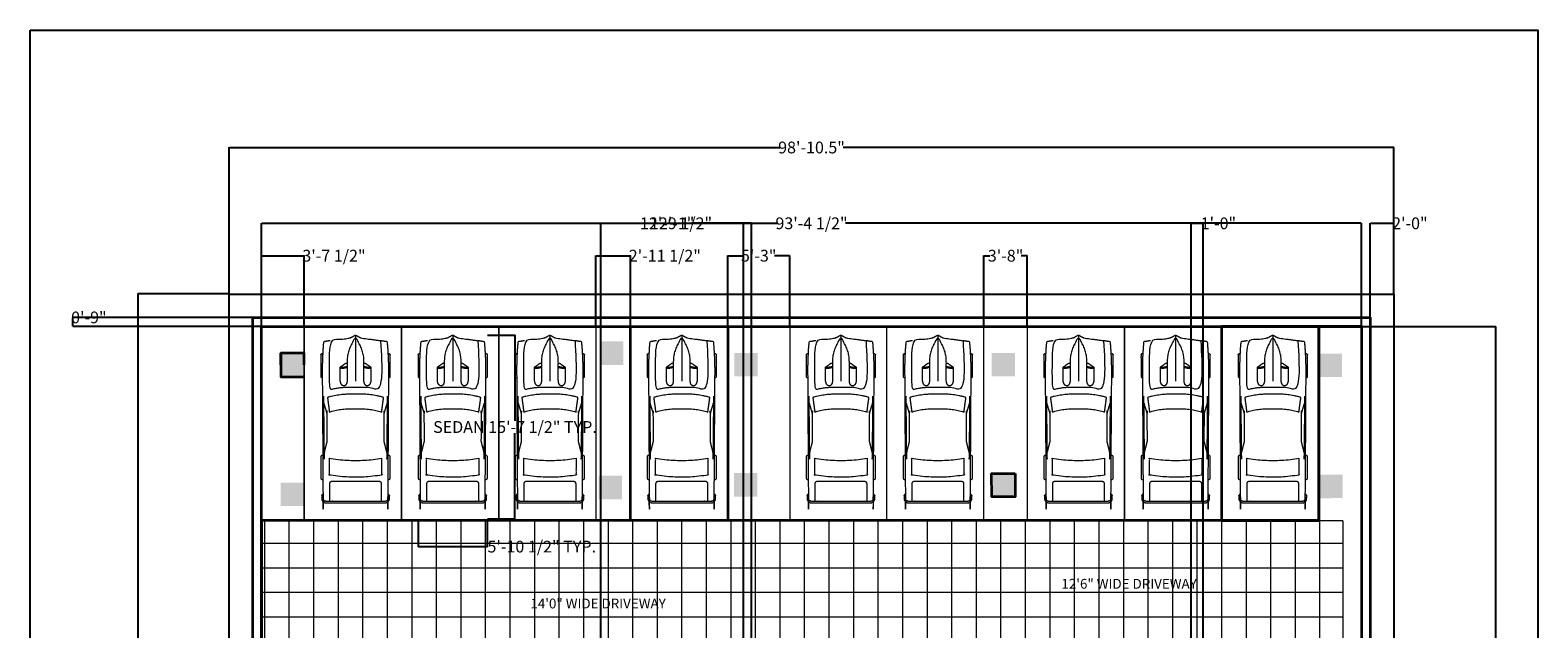
# Model space of a CAD drawing. Units: inches. Extents: x 48986 to 50522, y 132527 to 134098.
# Tile 4 of 4: x 48986 to 50522, y 133488 to 134098. Entities that reach past the tile are written whole.
import ezdxf

# ---------------------------------------------------------------- set-up
doc = ezdxf.new("R2010")
doc.units = ezdxf.units.IN
doc.header["$MEASUREMENT"] = 0
for name, color, linetype, lineweight in [('A-ANNO-DIMS', 2, 'Continuous', 18), ('A-ANNO-TEXT', 7, 'Continuous', 18), ('A-ANNO-TTLB', 7, 'Continuous', 25), ('A-COLS-PATT', 215, 'Continuous', 13), ('A-EQPM-VEHC', 8, 'Continuous', 13), ('A-FLOR-PATT', 94, 'Continuous', 9), ('A-FLOR-PKNG', 140, 'Continuous', 18), ('C-PROP', 160, 'Continuous', 25), ('COLUMNS', 211, 'Continuous', 35), ('WALLS', 140, 'Continuous', 35)]:
    doc.layers.add(name, color=color, linetype=linetype, lineweight=lineweight)
doc.styles.get("Standard").update_dxf_attribs({"font": 'arial.ttf'})
doc.dimstyles.get("Standard").update_dxf_attribs({"dimtxt": 12, "dimasz": 0.18, "dimexe": 0.18, "dimexo": 0.0625, "dimgap": 0.09, "dimtad": 0, "dimtih": 1, "dimtoh": 1, "dimdec": 1, "dimzin": 0, "dimdsep": 46, "dimlunit": 3, "dimtxsty": 'Standard', "dimcen": 0.09, "dimadec": 0, "dimazin": 0, "dimtfac": 1, "dimtdec": 1, "dimtofl": 0, "dimtmove": 0, "dimatfit": 3, "dimfxl": 1, "dimtolj": 1, "dimtzin": 0, "dimarcsym": 0})

# ---------------------------------------------------------------- blocks, each defined once
blk = doc.blocks.new('*D2')
at = {"layer": 'A-ANNO-DIMS', "color": 0, "lineweight": -2, "transparency": 16777216}
for p, q in [((49188.8, 133829.1), (49188.8, 133978.6)), ((49189, 133978.4), (49749.7, 133978.4)), ((50375.1, 133978.4), (49814.4, 133978.4)), ((50375.3, 133829.1), (50375.3, 133978.6))]:
    blk.add_line(p, q, dxfattribs=at)
at = {"layer": 'A-ANNO-DIMS', "color": 0, "transparency": 16777216}
for points in [[(49189, 133978.4), (49189, 133978.4), (49188.8, 133978.4)], [(50375.1, 133978.4), (50375.1, 133978.4), (50375.3, 133978.4)]]:
    blk.add_solid(points, dxfattribs=at)
at = {"layer": 'Defpoints', "color": 0, "transparency": 16777216}
for p in [(50375.3, 133978.4), (49188.8, 133829.1), (50375.3, 133829.1)]:
    blk.add_point(p, dxfattribs=at)
at = {"layer": 'A-ANNO-DIMS', "color": 0, "transparency": 16777216, "insert": (49782, 133978.4), "char_height": 12, "attachment_point": 5}
blk.add_mtext('\\A1;98\'-10.5"', dxfattribs=at)
blk = doc.blocks.new('*D3')
at = {"layer": 'A-ANNO-DIMS', "color": 0, "lineweight": -2, "transparency": 16777216}
for p, q in [((49188.7, 133829.1), (49095.4, 133829.1)), ((49095.6, 133828.9), (49095.6, 133304.8)), ((49095.6, 132768.2), (49095.6, 133292.3)), ((49188.7, 132768.1), (49095.4, 132768.1))]:
    blk.add_line(p, q, dxfattribs=at)
at = {"layer": 'A-ANNO-DIMS', "color": 0, "transparency": 16777216}
for points in [[(49095.6, 133828.9), (49095.6, 133828.9), (49095.6, 133829.1)], [(49095.6, 132768.2), (49095.6, 132768.2), (49095.6, 132768.1)]]:
    blk.add_solid(points, dxfattribs=at)
at = {"layer": 'Defpoints', "color": 0, "transparency": 16777216}
for p in [(49188.8, 133829.1), (49095.6, 132768.1), (49188.8, 132768.1)]:
    blk.add_point(p, dxfattribs=at)
at = {"layer": 'A-ANNO-DIMS', "color": 0, "transparency": 16777216, "insert": (49095.6, 133298.6), "char_height": 12, "attachment_point": 5}
blk.add_mtext('\\A1;88\'-5.0"', dxfattribs=at)
blk = doc.blocks.new('CAR-SEDAN-PLAN')
for p, q in [((35.3, 177.5), (35.3, 130.6)), ((25.7, 8.4), (44.8, 8.4))]:
    blk.add_line(p, q)
for centre, major_axis, start_param, end_param in [((19.9, 164.6), (-24.9, 0), 1.564964, 1.848039), ((50.7, 164.6), (24.9, 0), 4.435146, 4.718221)]:
    blk.add_ellipse(centre, major_axis=major_axis, ratio=0.842304, start_param=start_param, end_param=end_param)
for points, weights, knots in [([(9.6, 171.8), (6.2, 171.2), (2.7, 170.6), (1.4, 156), (1.4, 141.3)], [1, 0.999923835344, 1, 0.999337806115, 1], [0, 0, 0, 0.02468451, 0.02468451, 0.0974728, 0.0974728, 0.0974728]), ([(60.9, 171.8), (56.4, 172.5), (51.9, 173.1), (46.3, 173.7), (40.8, 174.6), (38.2, 176), (35.7, 177.4), (35.3, 177.6), (34.9, 177.4), (32.3, 176), (29.7, 174.6), (24.2, 173.7), (18.7, 173.1), (14.2, 172.5), (9.6, 171.8), (7.9, 146.8), (9.2, 121.9), (17.2, 123.7), (25.5, 124.1), (35.3, 124.1), (45.1, 124.1), (53.3, 123.7), (61.3, 121.9), (62.7, 146.8), (60.9, 171.8)], [1, 0.999861960732, 1, 0.999699858145, 1, 1, 1, 0.835952709181, 1, 1, 1, 0.999699858145, 1, 0.999861960732, 1, 0.998625728423, 1, 0.994860280211, 1, 1, 1, 0.994860280211, 1, 0.998625728423, 1], [0, 0, 0, 0.033232, 0.033232, 0.082234, 0.082234, 1.082234, 1.082234, 2.244094, 2.244094, 3.244094, 3.244094, 3.293097, 3.293097, 3.326328, 3.326328, 3.431193, 3.431193, 3.634055, 3.634055, 4.634055, 4.634055, 4.836917, 4.836917, 4.941783, 4.941783, 4.941783]), ([(43.9, 145.6), (47.3, 144.7), (50.9, 144.8), (50.9, 138), (50.9, 131.3), (50.6, 126), (47.4, 125.7), (44.2, 125.4), (43.9, 130.6), (43.9, 140.6), (43.9, 150.5), (43.9, 163.6), (35.3, 174.4), (26.7, 163.6), (26.7, 150.5), (26.7, 140.6), (26.7, 130.6), (26.4, 125.4), (23.2, 125.7), (20, 126), (19.7, 131.3), (19.7, 138), (19.7, 144.8), (23.3, 144.7), (26.7, 145.6)], [1, 0.990000279832, 1, 1, 1, 0.735618766318, 1, 0.735618766318, 1, 1, 1, 0.956755789522, 1, 0.956755789522, 1, 1, 1, 0.735618766318, 1, 0.735618766318, 1, 1, 1, 0.990000279832, 1], [0, 0, 0, 0.283075, 0.283075, 1.283075, 1.283075, 2.771508, 2.771508, 4.259942, 4.259942, 5.259942, 5.259942, 5.85026, 5.85026, 6.440579, 6.440579, 7.440579, 7.440579, 8.929012, 8.929012, 10.417446, 10.417446, 11.417446, 11.417446, 11.700521, 11.700521, 11.700521]), ([(69.2, 141.3), (69.1, 156), (67.8, 170.6), (64.4, 171.2), (60.9, 171.8)], [1, 0.999337806115, 1, 0.999923835344, 1], [0, 0, 0, 0.07278829, 0.07278829, 0.0974728, 0.0974728, 0.0974728]), ([(1.9, 158.4), (1.6, 158.4), (1.3, 158.4), (0.8, 158.4), (0.4, 158.1), (0, 157.7), (0, 157.3), (0, 146.3), (0, 135.3), (0, 134.8), (0.4, 134.5), (0.8, 134.2), (1.3, 134.2), (1.4, 134.2), (1.4, 134.2)], [1, 1, 1, 0.923879532511, 1, 0.923879532511, 1, 1, 1, 0.923879532511, 1, 0.923879532511, 1, 1, 1], [0, 0, 0, 1, 1, 1.785398, 1.785398, 2.570796, 2.570796, 3.570796, 3.570796, 4.356194, 4.356194, 5.141593, 5.141593, 6.141593, 6.141593, 6.141593]), ([(69.2, 134.2), (69.2, 134.2), (69.2, 134.2), (69.8, 134.2), (70.2, 134.5), (70.6, 134.8), (70.6, 135.3), (70.6, 146.3), (70.6, 157.3), (70.6, 157.7), (70.2, 158.1), (69.8, 158.4), (69.2, 158.4), (69, 158.4), (68.7, 158.4)], [1, 1, 1, 0.923879532511, 1, 0.923879532511, 1, 1, 1, 0.923879532511, 1, 0.923879532511, 1, 1, 1], [0, 0, 0, 1, 1, 1.785398, 1.785398, 2.570796, 2.570796, 3.570796, 3.570796, 4.356194, 4.356194, 5.141593, 5.141593, 6.141593, 6.141593, 6.141593]), ([(1.4, 141.7), (1.2, 76.1), (2.2, 10.6), (2.2, 8.4), (4.9, 8.4), (35.3, 8.4), (65.7, 8.4), (68.3, 8.4), (68.4, 10.6), (69.4, 76.1), (69.2, 141.7)], [1, 0.999967219517, 1, 0.711827418646, 1, 1, 1, 0.711827418646, 1, 0.999967219517, 1], [0, 0, 0, 0.016194, 0.016194, 1.573593, 1.573593, 2.573593, 2.573593, 4.130993, 4.130993, 4.147187, 4.147187, 4.147187]), ([(26.7, 148.4), (25.9, 148.4), (25.2, 148.4), (24.9, 148.4), (24.7, 148.3), (22.2, 146.5), (19.7, 144.8)], [1, 1, 1, 0.940892222322, 1, 1, 1], [0, 0, 0, 1, 1, 1.691083, 1.691083, 2.691083, 2.691083, 2.691083]), ([(50.9, 144.8), (48.3, 146.5), (45.8, 148.3), (45.6, 148.4), (45.4, 148.4), (44.7, 148.4), (43.9, 148.4)], [1, 1, 1, 0.940892222322, 1, 1, 1], [0, 0, 0, 1, 1, 1.691083, 1.691083, 2.691083, 2.691083, 2.691083]), ([(6.5, 69.3), (4.7, 62.5), (3, 55.7), (2.7, 82.7), (2.7, 109.7), (4.5, 103.7), (6.4, 97.7), (6.3, 83.5), (6.5, 69.3)], [1, 1, 1, 0.999994429546, 1, 1, 1, 0.999987377106, 1], [0, 0, 0, 1, 1, 1.006676, 1.006676, 2.006676, 2.006676, 2.016725, 2.016725, 2.016725]), ([(61.9, 99.1), (52.7, 101.9), (43, 102.5), (35.3, 102.5), (27.6, 102.5), (17.8, 101.9), (8.7, 99.1), (7.7, 106.6), (6.7, 114), (16, 116.6), (25.7, 117.2), (35.3, 117.2), (44.8, 117.2), (54.6, 116.6), (63.9, 114), (62.9, 106.6), (61.9, 99.1)], [1, 0.991000078903, 1, 1, 1, 0.991000078903, 1, 1, 1, 0.991394232237, 1, 1, 1, 0.991394232237, 1, 1, 1], [0, 0, 0, 0.268529, 0.268529, 1.268529, 1.268529, 1.537057, 1.537057, 2.537057, 2.537057, 2.799631, 2.799631, 3.799631, 3.799631, 4.062205, 4.062205, 5.062205, 5.062205, 5.062205]), ([(64.1, 69.3), (64.2, 83.5), (64.2, 97.7), (66, 103.7), (67.9, 109.7), (67.8, 82.7), (67.6, 55.7), (65.8, 62.5), (64.1, 69.3)], [1, 0.999987377106, 1, 1, 1, 0.999994429546, 1, 1, 1], [0, 0, 0, 0.010049, 0.010049, 1.010049, 1.010049, 1.016725, 1.016725, 2.016725, 2.016725, 2.016725]), ([(1.7, 54.7), (1.5, 54.7), (1.3, 54.7), (0, 54.7), (0, 53.5), (0, 42.5), (0, 31.6), (0, 30.4), (1.3, 30.4), (1.6, 30.4), (1.9, 30.4)], [1, 1, 1, 0.707106781187, 1, 1, 1, 0.707106781187, 1, 1, 1], [0, 0, 0, 1, 1, 2.570796, 2.570796, 3.570796, 3.570796, 5.141593, 5.141593, 6.141593, 6.141593, 6.141593]), ([(61.9, 52), (35.3, 47.4), (8.7, 52), (8.7, 43.4), (8.7, 34.9), (35.3, 30.3), (61.9, 34.9), (61.9, 43.4), (61.9, 52)], [1, 0.979868494456, 1, 1, 1, 0.979868494456, 1, 1, 1], [0, 0, 0, 0.401989, 0.401989, 1.401989, 1.401989, 1.803978, 1.803978, 2.803978, 2.803978, 2.803978]), ([(68.6, 30.4), (68.9, 30.4), (69.2, 30.4), (69.8, 30.4), (70.2, 30.8), (70.6, 31.1), (70.6, 31.6), (70.6, 42.5), (70.6, 53.5), (70.6, 54), (70.2, 54.3), (69.8, 54.7), (69.2, 54.7), (69.1, 54.7), (68.9, 54.7)], [1, 1, 1, 0.923879532511, 1, 0.923879532511, 1, 1, 1, 0.923879532511, 1, 0.923879532511, 1, 1, 1], [0, 0, 0, 1, 1, 1.785398, 1.785398, 2.570796, 2.570796, 3.570796, 3.570796, 4.356194, 4.356194, 5.141593, 5.141593, 6.141593, 6.141593, 6.141593]), ([(61.9, 8.4), (61.9, 17.2), (61.9, 26), (61.9, 28.3), (59.2, 28.3), (35.3, 28.3), (11.3, 28.3), (8.7, 28.3), (8.7, 26), (8.7, 17.2), (8.7, 8.4)], [1, 1, 1, 0.707106781187, 1, 1, 1, 0.707106781187, 1, 1, 1], [0, 0, 0, 1, 1, 2.570796, 2.570796, 3.570796, 3.570796, 5.141593, 5.141593, 6.141593, 6.141593, 6.141593]), ([(2.1, 15.3), (0.7, 14.9), (0.8, 13.6), (0.8, 12.1), (0.8, 10.6), (0.9, 6.6), (5.6, 6.6), (35.3, 6.6), (65, 6.6), (69.7, 6.6), (69.8, 10.6), (69.8, 12.1), (69.8, 13.6), (69.8, 14.9), (68.4, 15.3)], [1, 0.807168985933, 1, 0.999999981995, 1, 0.711827418646, 1, 1, 1, 0.711827418646, 1, 0.999999981995, 1, 0.807168985459, 1], [0, 0, 0, 1.262912, 1.262912, 1.263291, 1.263291, 2.82069, 2.82069, 3.82069, 3.82069, 5.37809, 5.37809, 5.378469, 5.378469, 6.641381, 6.641381, 6.641381])]:
    blk.add_rational_spline(points, weights, degree=2, knots=knots)
blk = doc.blocks.new('PARKING-STALL-99X198')
blk.add_lwpolyline([(198, 0), (198, 99), (0, 99), (0, 0)], close=True)
blk = doc.blocks.new('*D11')
at = {"layer": 'A-ANNO-DIMS', "color": 0, "lineweight": -2, "transparency": 16777216}
for p, q in [((49451.8, 133787.2), (49480, 133787.2)), ((49479.9, 133787), (49479.9, 133699.8)), ((49479.9, 133599.9), (49479.9, 133687.2)), ((49451.8, 133599.8), (49480, 133599.8))]:
    blk.add_line(p, q, dxfattribs=at)
at = {"layer": 'A-ANNO-DIMS', "color": 0, "transparency": 16777216}
for points in [[(49479.8, 133787), (49479.9, 133787), (49479.9, 133787.2)], [(49479.8, 133599.9), (49479.9, 133599.9), (49479.9, 133599.8)]]:
    blk.add_solid(points, dxfattribs=at)
at = {"layer": 'Defpoints', "color": 0, "transparency": 16777216}
for p in [(49451.7, 133787.2), (49479.9, 133787.2), (49451.7, 133599.8)]:
    blk.add_point(p, dxfattribs=at)
at = {"layer": 'A-ANNO-DIMS', "color": 0, "transparency": 16777216, "insert": (49479.9, 133693.5), "char_height": 12, "attachment_point": 5}
blk.add_mtext('\\A1;SEDAN 15\'-7 1/2" TYP.', dxfattribs=at)
blk = doc.blocks.new('*D12')
at = {"layer": 'A-ANNO-DIMS', "color": 0, "lineweight": -2, "transparency": 16777216}
for p, q in [((49381.2, 133599.7), (49381.2, 133571.5)), ((49451.7, 133599.7), (49451.7, 133571.5)), ((49381.3, 133571.6), (49451.6, 133571.6)), ((49451.7, 133571.6), (49451.9, 133571.6))]:
    blk.add_line(p, q, dxfattribs=at)
at = {"layer": 'A-ANNO-DIMS', "color": 0, "transparency": 16777216}
for points in [[(49381.3, 133571.7), (49381.3, 133571.6), (49381.2, 133571.6)], [(49451.6, 133571.7), (49451.6, 133571.6), (49451.7, 133571.6)]]:
    blk.add_solid(points, dxfattribs=at)
at = {"layer": 'Defpoints', "color": 0, "transparency": 16777216}
for p in [(49381.2, 133599.8), (49451.7, 133599.8), (49451.7, 133571.6)]:
    blk.add_point(p, dxfattribs=at)
at = {"layer": 'A-ANNO-DIMS', "color": 0, "transparency": 16777216, "insert": (49507.2, 133571.6), "char_height": 12, "attachment_point": 5}
blk.add_mtext('\\A1;5\'-10 1/2" TYP.', dxfattribs=at)
blk = doc.blocks.new('*D25')
at = {"layer": 'A-ANNO-DIMS', "color": 0, "lineweight": -2, "transparency": 16777216}
for p, q in [((49221.8, 133796.1), (49221.8, 133901.3)), ((49222, 133901.1), (49747.4, 133901.1)), ((50342.1, 133901.1), (49816.7, 133901.1)), ((50342.3, 133796.1), (50342.3, 133901.3))]:
    blk.add_line(p, q, dxfattribs=at)
at = {"layer": 'A-ANNO-DIMS', "color": 0, "transparency": 16777216}
for points in [[(49222, 133901.1), (49222, 133901.1), (49221.8, 133901.1)], [(50342.1, 133901.1), (50342.1, 133901.1), (50342.3, 133901.1)]]:
    blk.add_solid(points, dxfattribs=at)
at = {"layer": 'Defpoints', "color": 0, "transparency": 16777216}
for p in [(50342.3, 133901.1), (49221.8, 133796.1), (50342.3, 133796.1)]:
    blk.add_point(p, dxfattribs=at)
at = {"layer": 'A-ANNO-DIMS', "color": 0, "transparency": 16777216, "insert": (49782, 133901.1), "char_height": 12, "attachment_point": 5}
blk.add_mtext('\\A1;93\'-4 1/2"', dxfattribs=at)
blk = doc.blocks.new('*D26')
at = {"layer": 'A-ANNO-DIMS', "color": 0, "lineweight": -2, "transparency": 16777216}
for p, q in [((50342.4, 133796.1), (50479.1, 133796.1)), ((50478.9, 133795.9), (50478.9, 133304.8)), ((50478.9, 132801.2), (50478.9, 133292.3)), ((50342.4, 132801.1), (50479.1, 132801.1))]:
    blk.add_line(p, q, dxfattribs=at)
at = {"layer": 'A-ANNO-DIMS', "color": 0, "transparency": 16777216}
for points in [[(50478.9, 133795.9), (50479, 133795.9), (50478.9, 133796.1)], [(50478.9, 132801.2), (50479, 132801.2), (50478.9, 132801.1)]]:
    blk.add_solid(points, dxfattribs=at)
at = {"layer": 'Defpoints', "color": 0, "transparency": 16777216}
for p in [(50342.3, 133796.1), (50342.3, 132801.1), (50478.9, 132801.1)]:
    blk.add_point(p, dxfattribs=at)
at = {"layer": 'A-ANNO-DIMS', "color": 0, "transparency": 16777216, "insert": (50478.9, 133298.6), "char_height": 12, "attachment_point": 5}
blk.add_mtext('\\A1;82\'-11"', dxfattribs=at)
blk = doc.blocks.new('*D32')
at = {"layer": 'A-ANNO-DIMS', "color": 0, "lineweight": -2, "transparency": 16777216}
for p, q in [((49221.8, 133796.1), (49221.8, 133868.3)), ((49222, 133868.1), (49265.1, 133868.1)), ((49265.3, 133796.1), (49265.3, 133868.3)), ((49265.3, 133868.1), (49265.5, 133868.1))]:
    blk.add_line(p, q, dxfattribs=at)
at = {"layer": 'A-ANNO-DIMS', "color": 0, "transparency": 16777216}
for points in [[(49222, 133868.1), (49222, 133868.1), (49221.8, 133868.1)], [(49265.1, 133868.1), (49265.1, 133868.1), (49265.3, 133868.1)]]:
    blk.add_solid(points, dxfattribs=at)
at = {"layer": 'Defpoints', "color": 0, "transparency": 16777216}
for p in [(49265.3, 133868.1), (49221.8, 133796.1), (49265.3, 133796.1)]:
    blk.add_point(p, dxfattribs=at)
at = {"layer": 'A-ANNO-DIMS', "color": 0, "transparency": 16777216, "insert": (49295.5, 133868.1), "char_height": 12, "attachment_point": 5}
blk.add_mtext('\\A1;3\'-7 1/2"', dxfattribs=at)
blk = doc.blocks.new('*D33')
at = {"layer": 'A-ANNO-DIMS', "color": 0, "lineweight": -2, "transparency": 16777216}
for p, q in [((49562.3, 133796.1), (49562.3, 133868.3)), ((49562.5, 133868.1), (49597.4, 133868.1)), ((49597.6, 133796.1), (49597.6, 133868.3)), ((49597.6, 133868.1), (49597.8, 133868.1))]:
    blk.add_line(p, q, dxfattribs=at)
at = {"layer": 'A-ANNO-DIMS', "color": 0, "transparency": 16777216}
for points in [[(49562.5, 133868.1), (49562.5, 133868.1), (49562.3, 133868.1)], [(49597.4, 133868.1), (49597.4, 133868.1), (49597.6, 133868.1)]]:
    blk.add_solid(points, dxfattribs=at)
at = {"layer": 'Defpoints', "color": 0, "transparency": 16777216}
for p in [(49597.6, 133868.1), (49562.3, 133796.1), (49597.6, 133796.1)]:
    blk.add_point(p, dxfattribs=at)
at = {"layer": 'A-ANNO-DIMS', "color": 0, "transparency": 16777216, "insert": (49632.6, 133868.1), "char_height": 12, "attachment_point": 5}
blk.add_mtext('\\A1;2\'-11 1/2"', dxfattribs=at)
blk = doc.blocks.new('*D34')
at = {"layer": 'A-ANNO-DIMS', "color": 0, "lineweight": -2, "transparency": 16777216}
for p, q in [((49696.6, 133796.1), (49696.6, 133868.3)), ((49696.8, 133868.1), (49712.2, 133868.1)), ((49759.6, 133868.1), (49744.2, 133868.1)), ((49759.8, 133796.1), (49759.8, 133868.3))]:
    blk.add_line(p, q, dxfattribs=at)
at = {"layer": 'A-ANNO-DIMS', "color": 0, "transparency": 16777216}
for points in [[(49696.8, 133868.1), (49696.8, 133868.1), (49696.6, 133868.1)], [(49759.6, 133868.1), (49759.6, 133868.1), (49759.8, 133868.1)]]:
    blk.add_solid(points, dxfattribs=at)
at = {"layer": 'Defpoints', "color": 0, "transparency": 16777216}
for p in [(49759.8, 133868.1), (49696.6, 133796.1), (49759.8, 133796.1)]:
    blk.add_point(p, dxfattribs=at)
at = {"layer": 'A-ANNO-DIMS', "color": 0, "transparency": 16777216, "insert": (49728.2, 133868.1), "char_height": 12, "attachment_point": 5}
blk.add_mtext('\\A1;5\'-3"', dxfattribs=at)
blk = doc.blocks.new('*D35')
at = {"layer": 'A-ANNO-DIMS', "color": 0, "lineweight": -2, "transparency": 16777216}
for p, q in [((49957.6, 133796.1), (49957.6, 133868.3)), ((49957.7, 133868.1), (49963.6, 133868.1)), ((50001.6, 133868.1), (49995.7, 133868.1)), ((50001.8, 133796.1), (50001.8, 133868.3))]:
    blk.add_line(p, q, dxfattribs=at)
at = {"layer": 'A-ANNO-DIMS', "color": 0, "transparency": 16777216}
for points in [[(49957.7, 133868.1), (49957.7, 133868.1), (49957.6, 133868.1)], [(50001.6, 133868.1), (50001.6, 133868.1), (50001.8, 133868.1)]]:
    blk.add_solid(points, dxfattribs=at)
at = {"layer": 'Defpoints', "color": 0, "transparency": 16777216}
for p in [(50001.8, 133868.1), (49957.6, 133796.1), (50001.8, 133796.1)]:
    blk.add_point(p, dxfattribs=at)
at = {"layer": 'A-ANNO-DIMS', "color": 0, "transparency": 16777216, "insert": (49979.7, 133868.1), "char_height": 12, "attachment_point": 5}
blk.add_mtext('\\A1;3\'-8"', dxfattribs=at)
blk = doc.blocks.new('*D36')
at = {"layer": 'A-ANNO-DIMS', "color": 0, "lineweight": -2, "transparency": 16777216}
for p, q in [((49567.4, 133427.1), (49567.4, 133901.3)), ((49567.5, 133901.1), (49609.9, 133901.1)), ((49720.5, 133901.1), (49678.2, 133901.1)), ((49720.7, 133427.1), (49720.7, 133901.3))]:
    blk.add_line(p, q, dxfattribs=at)
at = {"layer": 'A-ANNO-DIMS', "color": 0, "transparency": 16777216}
for points in [[(49567.5, 133901.1), (49567.5, 133901.1), (49567.4, 133901.1)], [(49720.5, 133901.1), (49720.5, 133901.1), (49720.7, 133901.1)]]:
    blk.add_solid(points, dxfattribs=at)
at = {"layer": 'Defpoints', "color": 0, "transparency": 16777216}
for p in [(49720.7, 133901.1), (49567.4, 133427), (49720.7, 133427)]:
    blk.add_point(p, dxfattribs=at)
at = {"layer": 'A-ANNO-DIMS', "color": 0, "transparency": 16777216, "insert": (49644, 133901.1), "char_height": 12, "attachment_point": 5}
blk.add_mtext('\\A1;12\'-9 1/2"', dxfattribs=at)
blk = doc.blocks.new('*D40')
at = {"layer": 'A-ANNO-DIMS', "color": 0, "lineweight": -2, "transparency": 16777216}
for p, q in [((49212.7, 133805.1), (49029.4, 133805.1)), ((49029.5, 133805.1), (49029.5, 133805.2)), ((49029.5, 133805.2), (49029.7, 133805.2)), ((49029.5, 133796.2), (49029.5, 133804.9)), ((49221.7, 133796.1), (49029.4, 133796.1))]:
    blk.add_line(p, q, dxfattribs=at)
at = {"layer": 'A-ANNO-DIMS', "color": 0, "transparency": 16777216}
for points in [[(49029.5, 133804.9), (49029.6, 133804.9), (49029.5, 133805.1)], [(49029.5, 133796.2), (49029.6, 133796.2), (49029.5, 133796.1)]]:
    blk.add_solid(points, dxfattribs=at)
at = {"layer": 'Defpoints', "color": 0, "transparency": 16777216}
for p in [(49029.5, 133805.1), (49212.8, 133805.1), (49221.8, 133796.1)]:
    blk.add_point(p, dxfattribs=at)
at = {"layer": 'A-ANNO-DIMS', "color": 0, "transparency": 16777216, "insert": (49045.8, 133805.2), "char_height": 12, "attachment_point": 5}
blk.add_mtext('\\A1;0\'-9"', dxfattribs=at)
blk = doc.blocks.new('*D41')
at = {"layer": 'A-ANNO-DIMS', "color": 0, "lineweight": -2, "transparency": 16777216}
for p, q in [((50351.3, 133805.1), (50351.3, 133901.3)), ((50351.5, 133901.1), (50375.1, 133901.1)), ((50375.3, 133829.1), (50375.3, 133901.3)), ((50375.3, 133901.1), (50375.5, 133901.1))]:
    blk.add_line(p, q, dxfattribs=at)
at = {"layer": 'A-ANNO-DIMS', "color": 0, "transparency": 16777216}
for points in [[(50351.5, 133901.1), (50351.5, 133901.1), (50351.3, 133901.1)], [(50375.1, 133901.1), (50375.1, 133901.1), (50375.3, 133901.1)]]:
    blk.add_solid(points, dxfattribs=at)
at = {"layer": 'Defpoints', "color": 0, "transparency": 16777216}
for p in [(50375.3, 133901.1), (50375.3, 133829.1), (50351.3, 133805.1)]:
    blk.add_point(p, dxfattribs=at)
at = {"layer": 'A-ANNO-DIMS', "color": 0, "transparency": 16777216, "insert": (50391.6, 133901.1), "char_height": 12, "attachment_point": 5}
blk.add_mtext('\\A1;2\'-0"', dxfattribs=at)
blk = doc.blocks.new('*D42')
at = {"layer": 'A-ANNO-DIMS', "color": 0, "lineweight": -2, "transparency": 16777216}
for p, q in [((50168.9, 133343.1), (50168.9, 133901.3)), ((50169, 133901.1), (50180.7, 133901.1)), ((50180.9, 133343.1), (50180.9, 133901.3)), ((50180.9, 133901.1), (50181, 133901.1))]:
    blk.add_line(p, q, dxfattribs=at)
at = {"layer": 'A-ANNO-DIMS', "color": 0, "transparency": 16777216}
for points in [[(50169, 133901.1), (50169, 133901.1), (50168.9, 133901.1)], [(50180.7, 133901.1), (50180.7, 133901.1), (50180.9, 133901.1)]]:
    blk.add_solid(points, dxfattribs=at)
at = {"layer": 'Defpoints', "color": 0, "transparency": 16777216}
for p in [(50180.9, 133901.1), (50168.9, 133343.1), (50180.9, 133343.1)]:
    blk.add_point(p, dxfattribs=at)
at = {"layer": 'A-ANNO-DIMS', "color": 0, "transparency": 16777216, "insert": (50196.5, 133901.1), "char_height": 12, "attachment_point": 5}
blk.add_mtext('\\A1;1\'-0"', dxfattribs=at)
blk = doc.blocks.new('*D44')
at = {"layer": 'A-ANNO-DIMS', "color": 0, "lineweight": -2, "transparency": 16777216}
for p, q in [((49567.4, 132837.1), (49567.4, 133901.3)), ((49567.5, 133901.1), (49619.8, 133901.1)), ((49712.4, 133901.1), (49660.1, 133901.1)), ((49712.6, 132837.1), (49712.6, 133901.3))]:
    blk.add_line(p, q, dxfattribs=at)
at = {"layer": 'A-ANNO-DIMS', "color": 0, "transparency": 16777216}
for points in [[(49567.5, 133901.1), (49567.5, 133901.1), (49567.4, 133901.1)], [(49712.4, 133901.1), (49712.4, 133901.1), (49712.6, 133901.1)]]:
    blk.add_solid(points, dxfattribs=at)
at = {"layer": 'Defpoints', "color": 0, "transparency": 16777216}
for p in [(49712.6, 133901.1), (49567.4, 132837.1), (49712.6, 132837.1)]:
    blk.add_point(p, dxfattribs=at)
at = {"layer": 'A-ANNO-DIMS', "color": 0, "transparency": 16777216, "insert": (49640, 133901.1), "char_height": 12, "attachment_point": 5}
blk.add_mtext('\\A1;12\'-1"', dxfattribs=at)

msp = doc.modelspace()

# ---------------------------------------------------------------- hatches: boundary and pattern name
at = {"layer": 'A-COLS-PATT'}
h = msp.add_hatch(color=256, dxfattribs=at)
h.dxf.hatch_style = 1
h.paths.add_polyline_path([(49265.29, 133768.81), (49253.29, 133768.81), (49241.29, 133768.81), (49241.29, 133744.81), (49253.29, 133744.81), (49265.29, 133744.81)])
h = msp.add_hatch(color=256, dxfattribs=at)
h.dxf.hatch_style = 1
h.paths.add_polyline_path([(49265.29, 133768.81), (49253.29, 133768.81), (49253.29, 133756.81), (49265.29, 133756.81)])
h.paths.add_polyline_path([(49265.29, 133624.83), (49253.29, 133624.83), (49253.29, 133612.83), (49265.29, 133612.83)])
h.paths.add_polyline_path([(49578.45, 133768.81), (49566.45, 133768.81), (49566.45, 133756.81), (49578.45, 133756.81)])
h.paths.add_polyline_path([(49577.26, 133632.25), (49565.26, 133632.25), (49565.26, 133620.25), (49577.26, 133620.25)])
h.paths.add_polyline_path([(49715.36, 133768.81), (49703.36, 133768.81), (49703.36, 133756.81), (49715.36, 133756.81)])
h.paths.add_polyline_path([(49715.36, 133634.81), (49703.36, 133634.81), (49703.36, 133622.81), (49715.36, 133622.81)])
h.paths.add_polyline_path([(49977.6, 133768.81), (49965.6, 133768.81), (49965.6, 133756.81), (49977.6, 133756.81)])
h.paths.add_polyline_path([(49977.6, 133634.81), (49965.6, 133634.81), (49965.6, 133622.81), (49977.6, 133622.81)])
h.paths.add_polyline_path([(50310.67, 133768.05), (50298.79, 133768.05), (50298.79, 133756.05), (50310.67, 133756.05)])
h.paths.add_polyline_path([(50311.31, 133632.92), (50299.31, 133632.92), (50299.31, 133620.92), (50311.31, 133620.92)])
h = msp.add_hatch(color=256, dxfattribs=at)
h.dxf.hatch_style = 1
h.paths.add_polyline_path([(49590.43, 133780.81), (49578.43, 133780.81), (49566.43, 133780.81), (49566.43, 133756.81), (49578.43, 133756.81), (49590.43, 133756.81)])
h = msp.add_hatch(color=256, dxfattribs=at)
h.dxf.hatch_style = 1
h.paths.add_polyline_path([(49727.29, 133768.99), (49715.29, 133768.99), (49703.29, 133768.99), (49703.29, 133744.99), (49715.29, 133744.99), (49727.29, 133744.99)])
h = msp.add_hatch(color=256, dxfattribs=at)
h.dxf.hatch_style = 1
h.paths.add_polyline_path([(49989.44, 133769.07), (49977.44, 133769.07), (49965.44, 133769.07), (49965.44, 133745.07), (49977.44, 133745.07), (49989.44, 133745.07)])
h = msp.add_hatch(color=256, dxfattribs=at)
h.dxf.hatch_style = 1
h.paths.add_polyline_path([(50322.56, 133768.36), (50310.56, 133768.36), (50298.56, 133768.36), (50298.56, 133744.36), (50310.56, 133744.36), (50322.56, 133744.36)])
h = msp.add_hatch(color=256, dxfattribs=at)
h.dxf.hatch_style = 1
h.paths.add_polyline_path([(49726.9, 133646.48), (49714.9, 133646.48), (49702.9, 133646.48), (49702.9, 133622.48), (49714.9, 133622.48), (49726.9, 133622.48)])
h = msp.add_hatch(color=256, dxfattribs=at)
h.dxf.hatch_style = 1
h.paths.add_polyline_path([(49989.53, 133646.48), (49977.53, 133646.48), (49965.53, 133646.48), (49965.53, 133622.48), (49977.53, 133622.48), (49989.53, 133622.48)])
h = msp.add_hatch(color=256, dxfattribs=at)
h.dxf.hatch_style = 1
h.paths.add_polyline_path([(50322.96, 133644.98), (50310.96, 133644.98), (50298.96, 133644.98), (50298.96, 133620.98), (50310.96, 133620.98), (50322.96, 133620.98)])
h = msp.add_hatch(color=256, dxfattribs=at)
h.dxf.hatch_style = 1
h.paths.add_polyline_path([(49265.29, 133636.83), (49253.29, 133636.83), (49241.29, 133636.83), (49241.29, 133612.83), (49253.29, 133612.83), (49265.29, 133612.83)])
h = msp.add_hatch(color=256, dxfattribs=at)
h.dxf.hatch_style = 1
h.paths.add_polyline_path([(49589.05, 133643.94), (49577.05, 133643.94), (49565.05, 133643.94), (49565.05, 133619.94), (49577.05, 133619.94), (49589.05, 133619.94)])
at = {"layer": 'A-FLOR-PATT'}
h = msp.add_hatch(dxfattribs=at)
h.set_pattern_fill('NET', color=256, scale=200)
h.paths.add_polyline_path([(50323.33, 133597.94), (50298.79, 133598.06), (50199.79, 133598.06), (49957.56, 133598.06), (49597.63, 133598.06), (49221.79, 133598.06), (49221.79, 132801.06), (49253.29, 132801.06), (49253.29, 132832.63), (49251.14, 132832.63), (49251.14, 132842.53), (49253.29, 132842.53), (49253.29, 132956.08), (49251.14, 132956.08), (49251.14, 132965.97), (49253.29, 132965.97), (49253.29, 133105.3), (49251.14, 133105.3), (49251.14, 133115.2), (49253.29, 133115.2), (49253.29, 133143.75), (49253.29, 133153.65), (49253.29, 133244.43), (49251.14, 133244.43), (49251.14, 133254.33), (49253.29, 133254.33), (49253.29, 133283.54), (49253.29, 133293.44), (49253.29, 133335.08), (49251.14, 133335.08), (49248.66, 133335.08), (49248.66, 133344.97), (49251.14, 133344.97), (49253.29, 133344.97), (49253.29, 133387.65), (49253.29, 133397.55), (49253.29, 133425.06), (49253.29, 133426.99), (49420.79, 133426.99), (49423.36, 133426.99), (49423.36, 133344.97), (49425.09, 133344.97), (49425.09, 133335.08), (49423.36, 133335.08), (49423.36, 132813.06), (49567.36, 132813.06), (49567.36, 133229.31), (49567.36, 133241.64), (49567.36, 133265.64), (49567.36, 133335.08), (49567.36, 133344.97), (49567.36, 133361.98), (49567.36, 133385.98), (49567.36, 133426.99), (49591.36, 133426.99), (49690.36, 133426.99), (49817.62, 133426.99), (49817.62, 133427.11), (49841.62, 133427.11), (49995.88, 133426.99), (49995.88, 132801.06), (50139.88, 132801.06), (50139.88, 133259.08, -0.3612414), (50136.6, 133263.03, -0.3612414), (50139.88, 133266.99), (50139.88, 133448.06), (50303.12, 133448.06), (50303.12, 133472.06), (50323.33, 133472.06)])

# ---------------------------------------------------------------- linework, layer by layer
at = {"layer": 'A-ANNO-TTLB'}
msp.add_lwpolyline([(48985.99, 134098.01), (50521.96, 134098.01), (50521.96, 132528.75), (48985.99, 132528.75)], close=True, dxfattribs=at)
at = {"layer": 'A-FLOR-PKNG'}
msp.add_line((50298.79, 133598.06), (50298.79, 133598.06), dxfattribs=at)
for points in [[(49364.29, 133796.06), (49364.29, 133598.06), (49364.29, 133796.06), (49463.29, 133796.06), (49463.29, 133598.06), (49463.29, 133796.06), (49562.29, 133796.06), (49562.29, 133598.06), (49463.29, 133598.06), (49364.29, 133598.06), (49265.29, 133598.06), (49221.79, 133598.06)], [(49265.29, 133598.06), (49364.29, 133598.06), (49364.29, 133796.06), (49265.29, 133796.06), (49265.29, 133598.06), (49265.29, 133796.06), (49221.79, 133796.06)], [(50323.33, 133597.94), (50298.79, 133598.06), (50323.33, 133597.94), (50323.33, 133472.06), (50303.12, 133472.06), (50303.12, 133448.06), (50303.12, 133472.06), (50327.12, 133472.06), (50327.12, 133448.06)]]:
    msp.add_lwpolyline(points, dxfattribs=at)
at = {"layer": 'C-PROP'}
msp.add_line((49188.79, 133829.06), (50375.29, 133829.06), dxfattribs=at)
msp.add_lwpolyline([(49188.79, 133829.06), (50375.29, 133829.06), (50375.29, 132768.06), (49188.79, 132768.06)], close=True, dxfattribs=at)
at = {"layer": 'COLUMNS'}
msp.add_line((49241.29, 133756.81), (49241.29, 133768.81), dxfattribs=at)
msp.add_lwpolyline([(49265.29, 133756.81), (49265.29, 133768.81), (49253.29, 133768.81), (49241.29, 133768.81), (49241.29, 133744.81), (49253.29, 133744.81), (49265.29, 133744.81)], dxfattribs=at)
msp.add_lwpolyline([(49989.64, 133646.08), (49989.64, 133622.44), (49965.6, 133622.44), (49965.43, 133646.08)], close=True, dxfattribs=at)
at = {"layer": 'WALLS'}
msp.add_lwpolyline([(49212.79, 133805.06), (50351.29, 133805.06), (50351.29, 132792.06), (49212.79, 132792.06)], close=True, dxfattribs=at)
msp.add_lwpolyline([(50342.29, 133796.06), (50342.29, 132801.06), (49221.79, 132801.06), (49221.79, 133796.06), (50342.29, 133796.06), (50298.79, 133796.06), (50298.79, 133598.06), (50298.79, 133796.06), (50199.79, 133796.06), (50199.79, 133598.06), (50298.79, 133598.06), (49957.56, 133598.06), (49597.63, 133598.06), (49597.63, 133796.06), (49696.63, 133796.06), (49696.63, 133598.06), (49597.63, 133598.06), (49221.79, 133598.06), (49221.79, 133426.99)], dxfattribs=at)

# ---------------------------------------------------------------- block references
at = {"layer": 'A-EQPM-VEHC'}
for p in [(49282.17, 133609.68), (49381.17, 133609.68), (49480.17, 133609.68), (49614.51, 133609.68), (49776.64, 133609.68), (49875.44, 133609.68), (50018.67, 133609.68), (50117.67, 133609.68), (50216.67, 133609.68)]:
    msp.add_blockref('CAR-SEDAN-PLAN', p, dxfattribs=at)
at = {"layer": 'A-FLOR-PKNG'}
for p, rotation in [((49759.76, 133796.06), 269.9999999999972), ((49858.56, 133796.06), 269.9999999999972), ((50001.79, 133796.06), 269.9999999999972), ((50100.79, 133796.06), 269.9999999999915)]:
    msp.add_blockref('PARKING-STALL-99X198', p, dxfattribs=dict(at, rotation=rotation))

# ---------------------------------------------------------------- texts
at = {"layer": 'A-ANNO-TEXT', "char_height": 10, "attachment_point": 1}
for s, width, insert in [('12\'6" WIDE DRIVEWAY', 234.0775, (50036.57, 133538.68)), ('14\'0" WIDE DRIVEWAY', 920.0829, (49495.59, 133518.59))]:
    msp.add_mtext_dynamic_manual_height_columns(s, width=width, gutter_width=1, heights=[0], dxfattribs=dict(at, insert=insert))

# ---------------------------------------------------------------- dimensions: what is measured, and where the dimension line sits
at = {"layer": 'A-ANNO-DIMS'}
for base, p1, p2, override, picture, middle in [((50375.29, 133978.39), (49188.79, 133829.06), (50375.29, 133829.06), {"dimclrd": 0, "dimclre": 0, "dimclrt": 0}, '*D2', (49782.04, 133978.39)), ((50342.29, 133901.11), (49221.79, 133796.06), (50342.29, 133796.06), {"dimdec": 1, "dimlfac": 1, "dimrnd": 0, "dimzin": 1, "dimdsep": 46, "dimlunit": 4, "dimfrac": 2}, '*D25', (49782.04, 133901.11)), ((49720.71, 133901.1065), (49567.3578, 133426.9929), (49720.71, 133426.9929), {"dimdec": 1, "dimlfac": 1, "dimrnd": 0, "dimzin": 1, "dimdsep": 46, "dimlunit": 4, "dimfrac": 2}, '*D36', (49644.0339, 133901.1065)), ((49712.57, 133901.11), (49567.36, 132837.06), (49712.57, 132837.06), {"dimdec": 1, "dimlfac": 1, "dimrnd": 0, "dimzin": 1, "dimdsep": 46, "dimlunit": 4, "dimfrac": 2}, '*D44', (49639.96, 133901.11)), ((50180.85, 133901.11), (50168.85, 133343.06), (50180.85, 133343.06), {"dimdec": 1, "dimlfac": 1, "dimrnd": 0, "dimzin": 1, "dimdsep": 46, "dimlunit": 4, "dimfrac": 2}, '*D42', (50196.51, 133901.11)), ((50375.29, 133901.11), (50351.29, 133805.06), (50375.29, 133829.06), {"dimdec": 1, "dimlfac": 1, "dimrnd": 0, "dimzin": 1, "dimdsep": 46, "dimlunit": 4, "dimfrac": 2}, '*D41', (50391.61, 133901.11)), ((49265.29, 133868.11), (49221.79, 133796.06), (49265.29, 133796.06), {"dimdec": 1, "dimlfac": 1, "dimrnd": 0, "dimzin": 1, "dimdsep": 46, "dimlunit": 4, "dimfrac": 2}, '*D32', (49295.49, 133868.11)), ((49597.63, 133868.11), (49562.29, 133796.06), (49597.63, 133796.06), {"dimdec": 1, "dimlfac": 1, "dimrnd": 0, "dimzin": 1, "dimdsep": 46, "dimlunit": 4, "dimfrac": 2}, '*D33', (49632.59, 133868.11)), ((49759.76, 133868.11), (49696.63, 133796.06), (49759.76, 133796.06), {"dimdec": 1, "dimlfac": 1, "dimrnd": 0, "dimzin": 1, "dimdsep": 46, "dimlunit": 4, "dimfrac": 2}, '*D34', (49728.19, 133868.11)), ((50001.79, 133868.11), (49957.56, 133796.06), (50001.79, 133796.06), {"dimdec": 1, "dimlfac": 1, "dimrnd": 0, "dimzin": 1, "dimdsep": 46, "dimlunit": 4, "dimfrac": 2}, '*D35', (49979.67, 133868.11))]:
    dim = msp.add_linear_dim(base=base, p1=p1, p2=p2, dimstyle='Standard', override=override, dxfattribs=at)
    dim.commit()
    dim.dimension.update_dxf_attribs({"geometry": picture, "text_midpoint": middle})
for base, p1, p2, override, picture, middle in [((49095.58, 132768.06), (49188.79, 133829.06), (49188.79, 132768.06), {"dimclrd": 0, "dimclre": 0, "dimclrt": 0}, '*D3', (49095.58, 133298.56)), ((49029.54, 133805.06), (49221.79, 133796.06), (49212.79, 133805.06), {"dimdec": 1, "dimlfac": 1, "dimrnd": 0, "dimzin": 1, "dimdsep": 46, "dimlunit": 4, "dimfrac": 2}, '*D40', (49045.76, 133805.24)), ((50478.94, 132801.06), (50342.29, 133796.06), (50342.29, 132801.06), {"dimdec": 1, "dimlfac": 1, "dimrnd": 0, "dimzin": 1, "dimdsep": 46, "dimlunit": 4, "dimfrac": 2}, '*D26', (50478.94, 133298.56))]:
    dim = msp.add_linear_dim(base=base, p1=p1, p2=p2, angle=90, dimstyle='Standard', override=override, dxfattribs=at)
    dim.commit()
    dim.dimension.update_dxf_attribs({"geometry": picture, "text_midpoint": middle})
dim = msp.add_linear_dim(base=(49479.8578, 133787.2105), p1=(49451.7398, 133599.7571), p2=(49451.7398, 133787.2105), angle=90, text='SEDAN <> TYP.', dimstyle='Standard', override={"dimdec": 1, "dimlfac": 1, "dimrnd": 0, "dimzin": 1, "dimdsep": 46, "dimlunit": 4, "dimfrac": 2}, dxfattribs=at)
dim.commit()
dim.dimension.update_dxf_attribs({"geometry": '*D11', "text_midpoint": (49479.8578, 133693.4838)})
dim = msp.add_linear_dim(base=(49451.74, 133571.64), p1=(49381.16, 133599.76), p2=(49451.74, 133599.76), text='<> TYP.', dimstyle='Standard', override={"dimdec": 1, "dimlfac": 1, "dimrnd": 0, "dimzin": 1, "dimdsep": 46, "dimlunit": 4, "dimfrac": 2}, dxfattribs=at)
dim.commit()
dim.dimension.update_dxf_attribs({"geometry": '*D12', "text_midpoint": (49507.23, 133571.64)})

doc.saveas('drawing.dxf')
